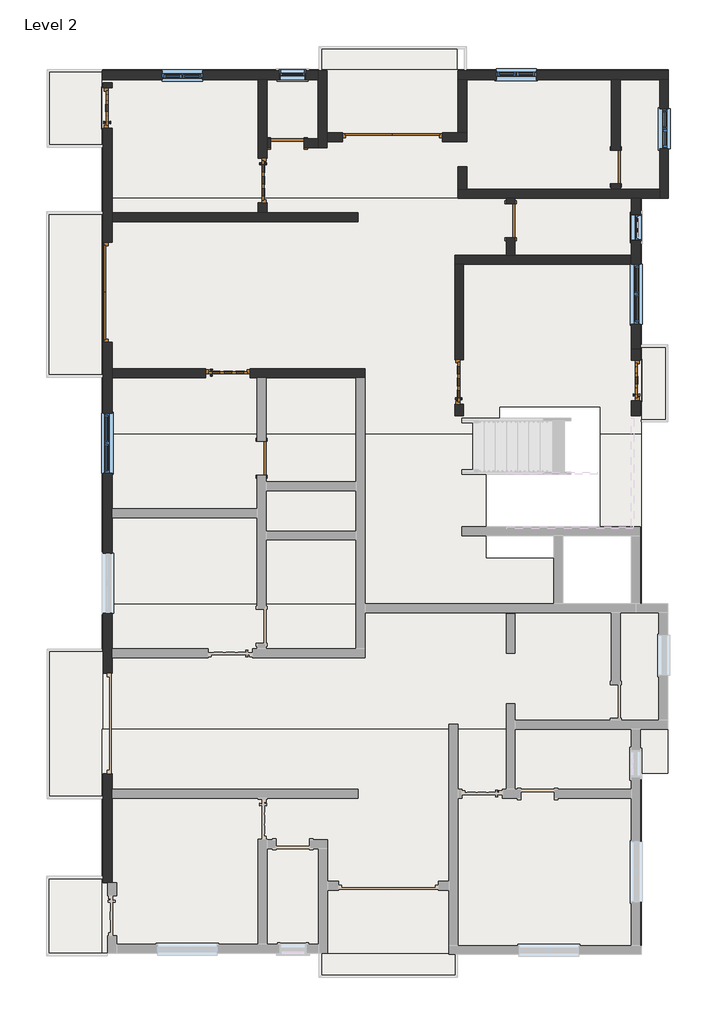
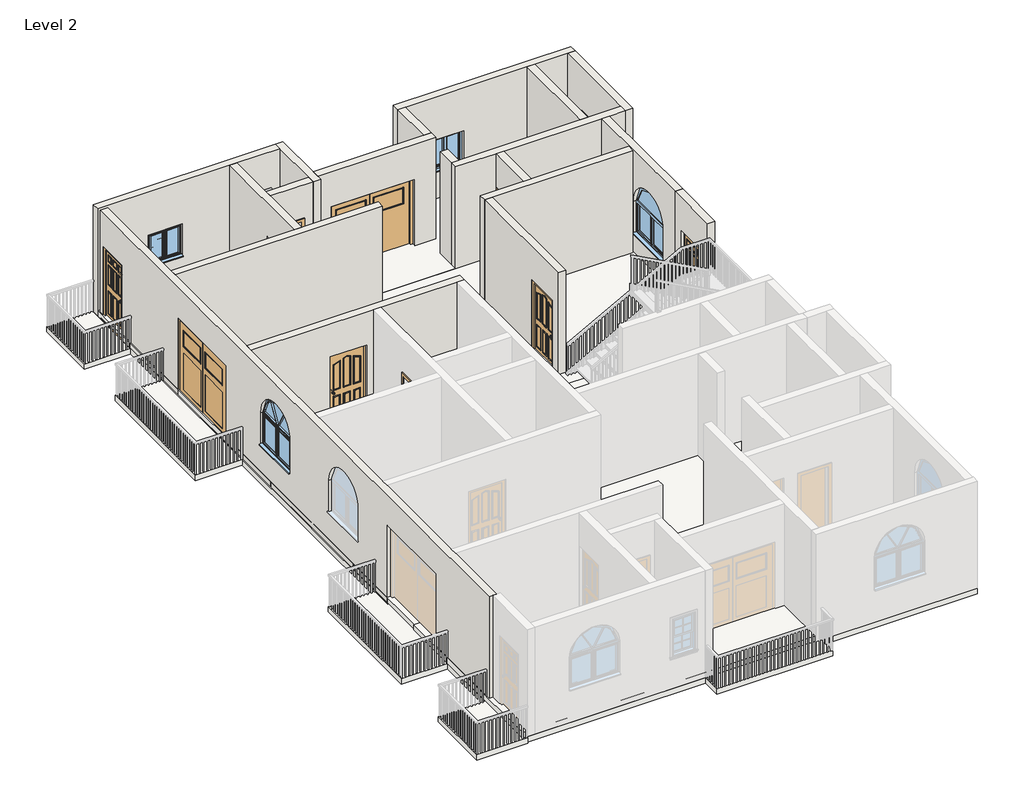
# One storey, part 2 of 7: 19 walls, 11 doors, 10 slabs, 7 windows, 5 roofs.
"""IFC4 building model written with IfcOpenShell, lengths in millimetres."""

from ifc_helpers import new_model, si_unit, point, frame, frame_2d, origin, place, context, project, spatial, polyline, circle_curve, trimmed, segment, composite_curve, outline, extrude, faceted_brep, transform, mapped, element, save
from ifc_brep_helpers import plane_surface, revolved_surface, advanced_brep
from components import doors_extsgl_5_910x2110mm_99758a98, doors_extsgl_5_910x2110mm_d3ca6061, doors_extsgl_6_1010x2110mm_b93c615f, doors_extsgl_6_1010x2110mm_efbaf1af, doors_garage_timber_side_hung_glazing_2270x2050mm_ae99176d, doors_garage_timber_side_hung_glazing_2270x2200mm_badb7014, door_53b1b562, window_679d2811, windows_arched_1360x910mm_c5754810, windows_dbl_w_glazing_bars_910x910mm_41eba874

model = new_model("IFC4")

# Units and contexts
model_context = context("Model", 3, world=origin())
ifc_project = project(units=[si_unit("LENGTHUNIT", "METRE", prefix="MILLI")], contexts=[model_context])

# Site, building, storey
site = spatial("IfcSite", under=ifc_project)
building = spatial("IfcBuilding", under=site)
storey = spatial("IfcBuildingStorey", under=building, Name="Level 2", Elevation=3048.0)

# Doors
placement = place(None, origin())
doors_extsgl_5_910x2110mm_shape = doors_extsgl_5_910x2110mm_99758a98(model_context)
element("IfcDoor", 1, ObjectType="Doors_ExtSgl_5 : 910x2110mm", at=placement, inside=storey, context=model_context, shape_type="MappedRepresentation", body=[
    mapped(doors_extsgl_5_910x2110mm_shape, transform((5761.5890963, 2376.5107951, 3048.0), x_axis=(0.0, 1.0, 0.0), y_axis=(-1.0, 0.0, 0.0), z_axis=(0.0, 0.0, 1.0))),
])
doors_extsgl_5_910x2110mm_2_shape = doors_extsgl_5_910x2110mm_d3ca6061(model_context)
element("IfcDoor", 2, ObjectType="Doors_ExtSgl_5 : 910x2110mm", at=placement, inside=storey, context=model_context, shape_type="MappedRepresentation", body=[
    mapped(doors_extsgl_5_910x2110mm_2_shape, transform((-6229.2013636, 8553.74399, 3048.0), x_axis=(0.0, 1.0, 0.0), y_axis=(-1.0, 0.0, 0.0), z_axis=(0.0, 0.0, 1.0))),
])
doors_extsgl_6_1010x2110mm_shape = doors_extsgl_6_1010x2110mm_b93c615f(model_context)
doors_extsgl_6_1010x2110mm_2_shape = doors_extsgl_6_1010x2110mm_efbaf1af(model_context)
element("IfcDoor", 3, ObjectType="Doors_ExtSgl_6 : 1010x2110mm", at=placement, inside=storey, context=model_context, shape_type="MappedRepresentation", body=[
    mapped(doors_extsgl_6_1010x2110mm_shape, transform((-2709.3109037, 6913.1295584, 3048.0), x_axis=(0.0, -1.0, 0.0), y_axis=(1.0, 0.0, 0.0), z_axis=(0.0, 0.0, 1.0))),
    mapped(doors_extsgl_6_1010x2110mm_2_shape, transform((-2709.3109037, 6913.1295584, 3048.0), x_axis=(0.0, -1.0, 0.0), y_axis=(1.0, 0.0, 0.0), z_axis=(0.0, 0.0, 1.0))),
])
element("IfcDoor", 4, ObjectType="Doors_ExtSgl_6 : 1010x2110mm", at=placement, inside=storey, context=model_context, shape_type="MappedRepresentation", body=[
    mapped(doors_extsgl_6_1010x2110mm_shape, transform((1748.3890963, 2341.0628918, 3048.0), x_axis=(0.0, 1.0, 0.0), y_axis=(-1.0, 0.0, 0.0), z_axis=(0.0, 0.0, 1.0))),
    mapped(doors_extsgl_6_1010x2110mm_2_shape, transform((1748.3890963, 2341.0628918, 3048.0), x_axis=(0.0, 1.0, 0.0), y_axis=(-1.0, 0.0, 0.0), z_axis=(0.0, 0.0, 1.0))),
])
element("IfcDoor", 5, ObjectType="Doors_ExtSgl_6 : 1010x2110mm", at=placement, inside=storey, context=model_context, shape_type="MappedRepresentation", body=[
    mapped(doors_extsgl_6_1010x2110mm_shape, transform((-3496.7442371, 2544.2962251, 3048.0), x_axis=(1.0, 0.0, 0.0), y_axis=(0.0, 1.0, 0.0), z_axis=(0.0, 0.0, 1.0))),
    mapped(doors_extsgl_6_1010x2110mm_2_shape, transform((-3496.7442371, 2544.2962251, 3048.0), x_axis=(1.0, 0.0, 0.0), y_axis=(0.0, 1.0, 0.0), z_axis=(0.0, 0.0, 1.0))),
])
doors_garage_timber_side_hung_glazing_2270x2050mm_shape = doors_garage_timber_side_hung_glazing_2270x2050mm_ae99176d(model_context)
element("IfcDoor", 6, ObjectType="Doors_Garage_Timber_Side_Hung_Glazing : 2270x2050mm", at=placement, inside=storey, context=model_context, shape_type="MappedRepresentation", body=[
    mapped(doors_garage_timber_side_hung_glazing_2270x2050mm_shape, transform((237.0890963, 7890.9962251, 3048.0), x_axis=(1.0, 0.0, 0.0), y_axis=(0.0, 1.0, 0.0), z_axis=(0.0, 0.0, 1.0))),
])
doors_garage_timber_side_hung_glazing_2270x2200mm_shape = doors_garage_timber_side_hung_glazing_2270x2200mm_badb7014(model_context)
element("IfcDoor", 7, ObjectType="Doors_Garage_Timber_Side_Hung_Glazing : 2270x2200mm", at=placement, inside=storey, context=model_context, shape_type="MappedRepresentation", body=[
    mapped(doors_garage_timber_side_hung_glazing_2270x2200mm_shape, transform((-6229.2013636, 4373.0962251, 3048.0), x_axis=(0.0, -1.0, 0.0), y_axis=(1.0, 0.0, 0.0), z_axis=(0.0, 0.0, 1.0))),
])
door_shape = door_53b1b562(model_context)
element("IfcDoor", 8, ObjectType="Single-Flush : 30\" x 80\"", at=placement, inside=storey, context=model_context, shape_type="MappedRepresentation", body=[
    mapped(door_shape, transform((-2150.5109037, 7751.2962251, 3048.0), x_axis=(-1.0, 0.0, 0.0), y_axis=(0.0, -1.0, 0.0), z_axis=(0.0, 0.0, 1.0))),
])
element("IfcDoor", 9, ObjectType="Single-Flush : 30\" x 80\"", at=placement, inside=storey, context=model_context, shape_type="MappedRepresentation", body=[
    mapped(door_shape, transform((2916.7890963, 5998.6962251, 3048.0), x_axis=(0.0, 1.0, 0.0), y_axis=(-1.0, 0.0, 0.0), z_axis=(0.0, 0.0, 1.0))),
])
element("IfcDoor", 10, ObjectType="Single-Flush : 30\" x 80\"", at=placement, inside=storey, context=model_context, shape_type="MappedRepresentation", body=[
    mapped(door_shape, transform((-2734.7109037, 613.8962251, 3048.0), x_axis=(0.0, 1.0, 0.0), y_axis=(-1.0, 0.0, 0.0), z_axis=(0.0, 0.0, 1.0))),
])
element("IfcDoor", 11, ObjectType="Single-Flush : 30\" x 80\"", at=placement, inside=storey, context=model_context, shape_type="MappedRepresentation", body=[
    mapped(door_shape, transform((5304.3890963, 7217.8962251, 3048.0), x_axis=(0.0, 1.0, 0.0), y_axis=(-1.0, 0.0, 0.0), z_axis=(0.0, 0.0, 1.0))),
])

# Roofs
element("IfcRoof", 12, ObjectType="Generic - 12\"", at=placement, inside=storey, context=model_context, shape_type="SweptSolid", body=[
    extrude(outline(polyline([(-6354.2109037, 9427.2527313), (6498.1890963, 9427.2527313), (6498.1890963, 6506.6962251), (-6354.2109037, 6506.6962251), (-6354.2109037, 9427.2527313)])), frame((0.0, 0.0, 3048.0), z_axis=(0.0, 0.0, 1.0), x_axis=(1.0, 0.0, 0.0)), (0.0, 0.0, 1.0), 152.4),
])
element("IfcRoof", 13, ObjectType="Generic - 12\"", at=placement, inside=storey, context=model_context, shape_type="SweptSolid", body=[
    extrude(outline(polyline([(-6330.8013636, -2688.1037749), (6485.4890963, -2688.1037749), (6485.4890963, -6529.1251987), (-6330.8013636, -6529.1251987), (-6330.8013636, -2688.1037749)])), frame((0.0, 0.0, 3048.0), z_axis=(0.0, 0.0, 1.0), x_axis=(1.0, 0.0, 0.0)), (0.0, 0.0, 1.0), 152.4),
])
element("IfcRoof", 14, ObjectType="Generic - 12\"", at=placement, inside=storey, context=model_context, shape_type="SweptSolid", body=[
    extrude(outline(polyline([(-6354.2109037, -5532.9037749), (5863.1890963, -5532.9037749), (5863.1890963, -10612.9037749), (-6354.2109037, -10612.9037749), (-6354.2109037, -5532.9037749)])), frame((0.0, 0.0, 3048.0), z_axis=(0.0, 0.0, 1.0), x_axis=(1.0, 0.0, 0.0)), (0.0, 0.0, 1.0), 152.4),
])
element("IfcRoof", 15, ObjectType="Generic - 12\"", at=placement, inside=storey, context=model_context, shape_type="SweptSolid", body=[
    extrude(outline(polyline([(-6330.8013636, 1160.801054), (-6330.8013636, 6506.6962251), (5875.8890963, 6506.6962251), (5875.8890963, 1160.801054), (4949.8616623, 1160.801054), (4949.8616623, 1784.6684315), (2663.8616623, 1784.6684315), (2663.8616623, 1160.801054), (-6330.8013636, 1160.801054)])), frame((0.0, 0.0, 3048.0), z_axis=(0.0, 0.0, 1.0), x_axis=(1.0, 0.0, 0.0)), (0.0, 0.0, 1.0), 152.4),
])
element("IfcRoof", 16, ObjectType="Generic - 12\"", at=placement, inside=storey, context=model_context, shape_type="SweptSolid", body=[
    extrude(outline(polyline([(-6330.8013636, -2688.1037749), (-6330.8013636, 1160.801054), (2663.8616623, 1160.801054), (2663.8616623, 941.43649), (2352.8853127, 941.43649), (2352.8853127, -1649.36351), (4097.8890963, -1649.36351), (4097.8890963, -2688.1037749), (-6330.8013636, -2688.1037749)])), frame((0.0, 0.0, 3048.0), z_axis=(0.0, 0.0, 1.0), x_axis=(1.0, 0.0, 0.0)), (0.0, 0.0, 1.0), 152.4),
    extrude(outline(polyline([(5875.8890963, 1160.801054), (5875.8890963, -2688.1037749), (5659.9890963, -2688.1037749), (5659.9890963, -1138.7037749), (4791.2853127, -1138.7037749), (4791.2853127, -958.5315685), (4949.8616623, -958.5315685), (4949.8616623, 1160.801054), (5875.8890963, 1160.801054)])), frame((0.0, 0.0, 3048.0), z_axis=(0.0, 0.0, 1.0), x_axis=(1.0, 0.0, 0.0)), (0.0, 0.0, 1.0), 152.4),
])

# Slabs
element("IfcSlab", 17, ObjectType="Generic - 12\"", at=placement, inside=storey, context=model_context, shape_type="SweptSolid", body=[
    extrude(outline(polyline([(1694.4140963, 9948.3962251), (1694.4140963, -11133.6037749), (-1426.6109037, -11133.6037749), (-1426.6109037, 9948.3962251), (1694.4140963, 9948.3962251)])), frame((0.0, 0.0, 2895.6), z_axis=(0.0, 0.0, 1.0), x_axis=(1.0, 0.0, 0.0)), (0.0, 0.0, 1.0), 152.4),
])
element("IfcSlab", 18, ObjectType="Generic - 12\"", at=placement, inside=storey, context=model_context, shape_type="SweptSolid", body=[
    extrude(outline(polyline([(5875.8890963, 9402.2962251), (5875.8890963, -10638.3037749), (1722.9890963, -10638.3037749), (1722.9890963, 9402.2962251), (5875.8890963, 9402.2962251)]), holes=[polyline([(4097.8890963, -2688.1037749), (5659.9890963, -2688.1037749), (5659.9890963, -1138.7037749), (4791.2853127, -1138.7037749), (4791.2853127, -958.5315685), (4949.8616623, -958.5315685), (4949.8616623, 1784.6684315), (2663.8616623, 1784.6684315), (2663.8616623, 941.43649), (2352.8853127, 941.43649), (2352.8853127, -1649.36351), (4097.8890963, -1649.36351), (4097.8890963, -2688.1037749)])]), frame((0.0, 0.0, 2895.6), z_axis=(0.0, 0.0, 1.0), x_axis=(1.0, 0.0, 0.0)), (0.0, 0.0, 1.0), 152.4),
])
element("IfcSlab", 19, ObjectType="Generic - 12\"", at=placement, inside=storey, context=model_context, shape_type="SweptSolid", body=[
    extrude(outline(polyline([(6498.1890963, 9402.2962251), (6498.1890963, 6506.6962251), (5875.8890963, 6506.6962251), (5875.8890963, 9402.2962251), (6498.1890963, 9402.2962251)])), frame((0.0, 0.0, 2895.6), z_axis=(0.0, 0.0, 1.0), x_axis=(1.0, 0.0, 0.0)), (0.0, 0.0, 1.0), 152.4),
])
element("IfcSlab", 20, ObjectType="Generic - 12\"", at=placement, inside=storey, context=model_context, shape_type="SweptSolid", body=[
    extrude(outline(polyline([(6485.4890963, 3183.81308), (6485.4890963, 1439.3962251), (5863.1890963, 1439.3962251), (5863.1890963, 3183.81308), (6485.4890963, 3183.81308)])), frame((0.0, 0.0, 2895.6), z_axis=(0.0, 0.0, 1.0), x_axis=(1.0, 0.0, 0.0)), (0.0, 0.0, 1.0), 152.4),
])
element("IfcSlab", 21, ObjectType="Generic - 12\"", at=placement, inside=storey, context=model_context, shape_type="SweptSolid", body=[
    extrude(outline(polyline([(6485.4890963, -2688.1037749), (6485.4890963, -5532.9037749), (5863.1890963, -5532.9037749), (5863.1890963, -2688.1037749), (6485.4890963, -2688.1037749)])), frame((0.0, 0.0, 2895.6), z_axis=(0.0, 0.0, 1.0), x_axis=(1.0, 0.0, 0.0)), (0.0, 0.0, 1.0), 152.4),
])
element("IfcSlab", 22, ObjectType="Generic - 12\"", at=placement, inside=storey, context=model_context, shape_type="SweptSolid", body=[
    extrude(outline(polyline([(-6330.8013636, 9427.2527313), (-6330.8013636, 7667.1584215), (-7598.8109037, 7667.1584215), (-7598.8109037, 9427.2527313), (-6330.8013636, 9427.2527313)])), frame((0.0, 0.0, 2895.6), z_axis=(0.0, 0.0, 1.0), x_axis=(1.0, 0.0, 0.0)), (0.0, 0.0, 1.0), 152.4),
])
element("IfcSlab", 23, ObjectType="Generic - 12\"", at=placement, inside=storey, context=model_context, shape_type="SweptSolid", body=[
    extrude(outline(polyline([(-6330.8013636, 6201.8962251), (-6330.8013636, 2455.3962251), (-7614.6859037, 2455.3962251), (-7614.6859037, 6201.8962251), (-6330.8013636, 6201.8962251)])), frame((0.0, 0.0, 2895.6), z_axis=(0.0, 0.0, 1.0), x_axis=(1.0, 0.0, 0.0)), (0.0, 0.0, 1.0), 152.4),
])
element("IfcSlab", 24, ObjectType="Generic - 12\"", at=placement, inside=storey, context=model_context, shape_type="SweptSolid", body=[
    extrude(outline(polyline([(-6330.8013636, -3716.8037749), (-6330.8013636, -7105.2894702), (-7598.8109037, -7105.2894702), (-7598.8109037, -3716.8037749), (-6330.8013636, -3716.8037749)])), frame((0.0, 0.0, 2895.6), z_axis=(0.0, 0.0, 1.0), x_axis=(1.0, 0.0, 0.0)), (0.0, 0.0, 1.0), 152.4),
])
element("IfcSlab", 25, ObjectType="Generic - 12\"", at=placement, inside=storey, context=model_context, shape_type="SweptSolid", body=[
    extrude(outline(polyline([(-6243.0859037, -8868.0845215), (-6243.0859037, -10663.7037749), (-7614.6859037, -10663.7037749), (-7614.6859037, -8868.0845215), (-6243.0859037, -8868.0845215)])), frame((0.0, 0.0, 2895.6), z_axis=(0.0, 0.0, 1.0), x_axis=(1.0, 0.0, 0.0)), (0.0, 0.0, 1.0), 152.4),
])
element("IfcSlab", 26, ObjectType="Generic - 12\"", at=placement, inside=storey, context=model_context, shape_type="SweptSolid", body=[
    extrude(outline(polyline([(-1236.1109037, 9427.2527313), (-1236.1109037, -10612.9037749), (-6354.2109037, -10612.9037749), (-6354.2109037, 9427.2527313), (-1236.1109037, 9427.2527313)])), frame((0.0, 0.0, 2895.6), z_axis=(0.0, 0.0, 1.0), x_axis=(1.0, 0.0, 0.0)), (0.0, 0.0, 1.0), 152.4),
])

# Walls
element("IfcWall", 27, ObjectType="Generic - 9\" w", at=placement, inside=storey, context=model_context, shape_type="Brep", body=[
    faceted_brep([(1722.9890963, 9199.0962251, 3048.0), (1926.1890963, 9199.0962251, 3048.0), (5202.7890963, 9199.0962251, 3048.0), (5405.9890963, 9199.0962251, 3048.0), (6294.9890963, 9199.0962251, 3048.0), (6498.1890963, 9199.0962251, 3048.0), (6498.1890963, 9199.0962251, 6096.0), (6294.9890963, 9199.0962251, 6096.0), (5405.9890963, 9199.0962251, 6096.0), (5202.7890963, 9199.0962251, 6096.0), (1926.1890963, 9199.0962251, 6096.0), (1722.9890963, 9199.0962251, 6096.0), (2588.7890963, 9199.0962251, 4872.4), (3498.7890963, 9199.0962251, 4872.4), (3498.7890963, 9199.0962251, 3962.4), (2588.7890963, 9199.0962251, 3962.4), (1722.9890963, 9402.2962251, 3048.0), (1722.9890963, 9402.2962251, 6096.0), (6498.1890963, 9402.2962251, 6096.0), (6498.1890963, 9402.2962251, 3048.0), (2588.7890963, 9402.2962251, 4872.4), (2588.7890963, 9402.2962251, 3962.4), (3498.7890963, 9402.2962251, 3962.4), (3498.7890963, 9402.2962251, 4872.4)], [[[0, 1, 2, 3, 4, 5, 6, 7, 8, 9, 10, 11], [12, 13, 14, 15]], [[16, 17, 18, 19], [20, 21, 22, 23]], [[5, 4, 3, 2, 1, 0, 16, 19]], [[11, 10, 9, 8, 7, 6, 18, 17]], [[0, 11, 17, 16]], [[6, 5, 19, 18]], [[21, 20, 12, 15]], [[22, 21, 15, 14]], [[23, 22, 14, 13]], [[20, 23, 13, 12]]]),
])
element("IfcWall", 28, ObjectType="Generic - 9\" w", at=placement, inside=storey, context=model_context, shape_type="SweptSolid", body=[
    extrude(outline(polyline([(6506.6962251, 3048.0), (3087.7441284, 3048.0), (3087.7441284, 6096.0), (6506.6962251, 6096.0), (6506.6962251, 3048.0)]), holes=[polyline([(6151.0962251, 5029.2), (5541.4962251, 5029.2), (5541.4962251, 3962.4), (6151.0962251, 3962.4), (6151.0962251, 5029.2)]), composite_curve([segment(polyline([(5016.7786331, 3733.6617803), (5016.7786331, 4643.6617803)]), True, "CONTINUOUS"), segment(trimmed(circle_curve(frame_2d((4336.7786331, 4643.6617803)), 680.0), [point((5016.7786331, 4643.6617803))], [point((3656.7786331, 4643.6617803))], True, "CARTESIAN"), True, "CONTINUOUS"), segment(polyline([(3656.7786331, 4643.6617803), (3656.7786331, 3733.6617803), (5016.7786331, 3733.6617803)]), True, "CONTINUOUS")], self_intersect=False)]), frame((5659.9890963, 0.0, 0.0), z_axis=(1.0, 0.0, 0.0), x_axis=(0.0, 1.0, 0.0)), (0.0, 0.0, 1.0), 203.2),
])
element("IfcWall", 29, ObjectType="Generic - 9\" w", at=placement, inside=storey, context=model_context, shape_type="AdvancedBrep", body=[
    advanced_brep(
    [(-6330.8013636, 3238.0962251, 3048.0), (-6330.8013636, -4267.1251987, 3048.0), (-6330.8013636, -4267.1251987, 5248.0), (-6330.8013636, -6537.1251987, 5248.0), (-6330.8013636, -6537.1251987, 3048.0), (-6330.8013636, -9007.7845215, 3048.0), (-6330.8013636, -9007.7845215, 6096.0), (-6330.8013636, 9129.8816143, 6096.0), (-6330.8013636, 9129.8816143, 3048.0), (-6330.8013636, 9008.7773233, 3048.0), (-6330.8013636, 9008.7773233, 5158.0), (-6330.8013636, 8098.7773233, 5158.0), (-6330.8013636, 8098.7773233, 3048.0), (-6330.8013636, 5508.0962251, 3048.0), (-6330.8013636, 5508.0962251, 5248.0), (-6330.8013636, 3238.0962251, 5248.0), (-6330.8013636, 276.7962251, 3962.4), (-6330.8013636, 1636.7962251, 3962.4), (-6330.8013636, 1636.7962251, 4872.4), (-6330.8013636, 276.7962251, 4872.4), (-6330.8013636, -1538.2037749, 3962.4), (-6330.8013636, -1538.2037749, 4872.4), (-6330.8013636, -2898.2037749, 4872.4), (-6330.8013636, -2898.2037749, 3962.4), (-6127.6013636, -4267.1251987, 5248.0), (-6127.6013636, -4267.1251987, 3048.0), (-6127.6013636, -3907.3037749, 3048.0), (-6127.6013636, -3704.1037749, 3048.0), (-6127.6013636, -732.3037749, 3048.0), (-6127.6013636, -529.1037749, 3048.0), (-6127.6013636, 2442.6962251, 3048.0), (-6127.6013636, 2645.8962251, 3048.0), (-6127.6013636, 3238.0962251, 3048.0), (-6127.6013636, 3238.0962251, 5248.0), (-6127.6013636, 5508.0962251, 5248.0), (-6127.6013636, 5508.0962251, 3048.0), (-6127.6013636, 5973.2962251, 3048.0), (-6127.6013636, 6176.4962251, 3048.0), (-6127.6013636, 8098.7773233, 3048.0), (-6127.6013636, 8098.7773233, 5158.0), (-6127.6013636, 9008.7773233, 5158.0), (-6127.6013636, 9008.7773233, 3048.0), (-6127.6013636, 9129.8816143, 3048.0), (-6127.6013636, 9129.8816143, 6096.0), (-6127.6013636, 6176.4962251, 6096.0), (-6127.6013636, 5973.2962251, 6096.0), (-6127.6013636, 2645.8962251, 6096.0), (-6127.6013636, 2442.6962251, 6096.0), (-6127.6013636, -529.1037749, 6096.0), (-6127.6013636, -732.3037749, 6096.0), (-6127.6013636, -3704.1037749, 6096.0), (-6127.6013636, -3907.3037749, 6096.0), (-6127.6013636, -6896.9466225, 6096.0), (-6127.6013636, -7100.1466225, 6096.0), (-6127.6013636, -9007.7845215, 6096.0), (-6127.6013636, -9007.7845215, 3048.0), (-6127.6013636, -7100.1466225, 3048.0), (-6127.6013636, -6896.9466225, 3048.0), (-6127.6013636, -6537.1251987, 3048.0), (-6127.6013636, -6537.1251987, 5248.0), (-6127.6013636, 276.7962251, 3962.4), (-6127.6013636, 276.7962251, 4872.4), (-6127.6013636, 1636.7962251, 4872.4), (-6127.6013636, 1636.7962251, 3962.4), (-6127.6013636, -1538.2037749, 3962.4), (-6127.6013636, -2898.2037749, 3962.4), (-6127.6013636, -2898.2037749, 4872.4), (-6127.6013636, -1538.2037749, 4872.4), (-6229.2013636, -9007.7845215, 3048.0), (-6229.2013636, -9007.7845215, 6096.0)],
    [
        (0, 1),
        (1, 2),
        (2, 3),
        (3, 4),
        (4, 5),
        (5, 6),
        (6, 7),
        (7, 8),
        (8, 9),
        (9, 10),
        (10, 11),
        (11, 12),
        (12, 13),
        (13, 14),
        (14, 15),
        (15, 0),
        (16, 17),
        (17, 18),
        (18, 19, circle_curve(frame((-6330.8013636, 956.7962251, 4872.4), z_axis=(1.0, 0.0, 0.0), x_axis=(0.0, 1.0, 0.0)), 680.0)),
        (19, 16),
        (20, 21),
        (21, 22, circle_curve(frame((-6330.8013636, -2218.2037749, 4872.4), z_axis=(1.0, 0.0, 0.0), x_axis=(0.0, -1.0, 0.0)), 680.0)),
        (22, 23),
        (23, 20),
        (24, 25),
        (25, 26),
        (26, 27),
        (27, 28),
        (28, 29),
        (29, 30),
        (30, 31),
        (31, 32),
        (32, 33),
        (33, 34),
        (34, 35),
        (35, 36),
        (36, 37),
        (37, 38),
        (38, 39),
        (39, 40),
        (40, 41),
        (41, 42),
        (42, 43),
        (43, 44),
        (44, 45),
        (45, 46),
        (46, 47),
        (47, 48),
        (48, 49),
        (49, 50),
        (50, 51),
        (51, 52),
        (52, 53),
        (53, 54),
        (54, 55),
        (55, 56),
        (56, 57),
        (57, 58),
        (58, 59),
        (59, 24),
        (60, 61),
        (61, 62, circle_curve(frame((-6127.6013636, 956.7962251, 4872.4), z_axis=(-1.0, 0.0, 0.0), x_axis=(0.0, 1.0, 0.0)), 680.0)),
        (62, 63),
        (63, 60),
        (64, 65),
        (65, 66),
        (66, 67, circle_curve(frame((-6127.6013636, -2218.2037749, 4872.4), z_axis=(-1.0, 0.0, 0.0), x_axis=(0.0, -1.0, 0.0)), 680.0)),
        (67, 64),
        (41, 9),
        (8, 42),
        (12, 38),
        (35, 13),
        (55, 68),
        (68, 5),
        (4, 58),
        (25, 1),
        (0, 32),
        (54, 69),
        (69, 6),
        (43, 7),
        (11, 39),
        (40, 10),
        (34, 14),
        (15, 33),
        (3, 59),
        (24, 2),
        (60, 16),
        (19, 61),
        (18, 62),
        (17, 63),
        (20, 64),
        (67, 21),
        (66, 22),
        (65, 23),
    ],
    [
        plane_surface(frame((-6330.8013636, 2442.6962251, 3048.0), z_axis=(-1.0, 0.0, 0.0), x_axis=(0.0, -1.0, 0.0))),
        plane_surface(frame((-6127.6013636, 2442.6962251, 3048.0), z_axis=(1.0, 0.0, 0.0), x_axis=(0.0, 1.0, 0.0))),
        plane_surface(frame((-6330.8013636, 9129.8816143, 3048.0), z_axis=(0.0, 0.0, -1.0), x_axis=(1.0, 0.0, 0.0))),
        plane_surface(frame((-6330.8013636, -9007.7845215, 3048.0), z_axis=(0.0, -1.0, 0.0), x_axis=(1.0, 0.0, 0.0))),
        plane_surface(frame((-6330.8013636, -9007.7845215, 6096.0), z_axis=(0.0, 0.0, 1.0), x_axis=(1.0, 0.0, 0.0))),
        plane_surface(frame((-6330.8013636, 9129.8816143, 6096.0), z_axis=(0.0, 1.0, 0.0), x_axis=(1.0, 0.0, 0.0))),
        plane_surface(frame((-6330.8013636, 8098.7773233, 5158.0), z_axis=(0.0, 1.0, 0.0), x_axis=(1.0, 0.0, 0.0))),
        plane_surface(frame((-6330.8013636, 9008.7773233, 3048.0), z_axis=(0.0, -1.0, 0.0), x_axis=(1.0, 0.0, 0.0))),
        plane_surface(frame((-6330.8013636, 9008.7773233, 5158.0), z_axis=(0.0, 0.0, -1.0), x_axis=(1.0, 0.0, 0.0))),
        plane_surface(frame((-6127.6013636, 5508.0962251, 5248.0), z_axis=(0.0, -1.0, 0.0), x_axis=(-1.0, 0.0, 0.0))),
        plane_surface(frame((-6127.6013636, 3238.0962251, 3048.0), z_axis=(0.0, 1.0, 0.0), x_axis=(-1.0, 0.0, 0.0))),
        plane_surface(frame((-6127.6013636, 3238.0962251, 5248.0), z_axis=(0.0, 0.0, -1.0), x_axis=(-1.0, 0.0, 0.0))),
        plane_surface(frame((-6330.8013636, -6537.1251987, 5248.0), z_axis=(0.0, 1.0, 0.0), x_axis=(1.0, 0.0, 0.0))),
        plane_surface(frame((-6330.8013636, -4267.1251987, 3048.0), z_axis=(0.0, -1.0, 0.0), x_axis=(1.0, 0.0, 0.0))),
        plane_surface(frame((-6330.8013636, -4267.1251987, 5248.0), z_axis=(0.0, 0.0, -1.0), x_axis=(1.0, 0.0, 0.0))),
        plane_surface(frame((-6127.6013636, 276.7962251, 3962.4), z_axis=(0.0, 1.0, 0.0), x_axis=(-1.0, 0.0, 0.0))),
        revolved_surface(polyline([(-6330.8013636, 1636.7962251, 4872.4), (-6127.6013636, 1636.7962251, 4872.4)]), (-6127.6013636, 956.7962251, 4872.4), (-1.0, 0.0, 0.0)),
        plane_surface(frame((-6127.6013636, 1636.7962251, 4872.4), z_axis=(0.0, -1.0, 0.0), x_axis=(-1.0, 0.0, 0.0))),
        plane_surface(frame((-6127.6013636, 1636.7962251, 3962.4), z_axis=(0.0, 0.0, 1.0), x_axis=(-1.0, 0.0, 0.0))),
        plane_surface(frame((-6330.8013636, -1538.2037749, 3962.4), z_axis=(0.0, -1.0, 0.0), x_axis=(1.0, 0.0, 0.0))),
        revolved_surface(polyline([(-6127.6013636, -2898.2037749, 4872.4), (-6330.8013636, -2898.2037749, 4872.4)]), (-6330.8013636, -2218.2037749, 4872.4), (1.0, 0.0, 0.0)),
        plane_surface(frame((-6330.8013636, -2898.2037749, 4872.4), z_axis=(0.0, 1.0, 0.0), x_axis=(1.0, 0.0, 0.0))),
        plane_surface(frame((-6330.8013636, -2898.2037749, 3962.4), z_axis=(0.0, 0.0, 1.0), x_axis=(1.0, 0.0, 0.0))),
    ],
    [
        (0, [[1, 2, 3, 4, 5, 6, 7, 8, 9, 10, 11, 12, 13, 14, 15, 16], [17, 18, 19, 20], [21, 22, 23, 24]]),
        (1, [[25, 26, 27, 28, 29, 30, 31, 32, 33, 34, 35, 36, 37, 38, 39, 40, 41, 42, 43, 44, 45, 46, 47, 48, 49, 50, 51, 52, 53, 54, 55, 56, 57, 58, 59, 60], [61, 62, 63, 64], [65, 66, 67, 68]]),
        (2, [[-42, 69, -9, 70]]),
        (2, [[-13, 71, -38, -37, -36, 72]]),
        (2, [[-58, -57, -56, 73, 74, -5, 75]]),
        (2, [[-32, -31, -30, -29, -28, -27, -26, 76, -1, 77]]),
        (3, [[-6, -74, -73, -55, 78, 79]]),
        (4, [[-7, -79, -78, -54, -53, -52, -51, -50, -49, -48, -47, -46, -45, -44, 80]]),
        (5, [[-8, -80, -43, -70]]),
        (6, [[-12, 81, -39, -71]]),
        (7, [[-10, -69, -41, 82]]),
        (8, [[-11, -82, -40, -81]]),
        (9, [[-35, 83, -14, -72]]),
        (10, [[-33, -77, -16, 84]]),
        (11, [[-34, -84, -15, -83]]),
        (12, [[-4, 85, -59, -75]]),
        (13, [[-2, -76, -25, 86]]),
        (14, [[-3, -86, -60, -85]]),
        (15, [[-61, 87, -20, 88]]),
        (16, [[-62, -88, -19, 89]]),
        (17, [[-63, -89, -18, 90]]),
        (18, [[-64, -90, -17, -87]]),
        (19, [[-21, 91, -68, 92]]),
        (20, [[-22, -92, -67, 93]]),
        (21, [[-23, -93, -66, 94]]),
        (22, [[-24, -94, -65, -91]]),
    ],
),
])
element("IfcWall", 30, ObjectType="Generic - 9\" w", at=placement, inside=storey, context=model_context, shape_type="SweptSolid", body=[
    extrude(outline(polyline([(3087.7441284, 3048.0), (2831.5441284, 3048.0), (2831.5441284, 5158.0), (1921.5441284, 5158.0), (1921.5441284, 3048.0), (1579.0962251, 3048.0), (1579.0962251, 6096.0), (3087.7441284, 6096.0), (3087.7441284, 3048.0)])), frame((5659.9890963, 0.0, 0.0), z_axis=(1.0, 0.0, 0.0), x_axis=(0.0, 1.0, 0.0)), (0.0, 0.0, 1.0), 203.2),
])
element("IfcWall", 31, ObjectType="Generic - 9\" w", at=placement, inside=storey, context=model_context, shape_type="Brep", body=[
    faceted_brep([(-1452.0109037, 9401.8527313, 3048.0), (-6354.2109037, 9401.8527313, 3048.0), (-6354.2109037, 9401.8527313, 6096.0), (-1452.0109037, 9401.8527313, 6096.0), (-4076.7609037, 9401.8527313, 4872.4), (-4986.7609037, 9401.8527313, 4872.4), (-4986.7609037, 9401.8527313, 3962.4), (-4076.7609037, 9401.8527313, 3962.4), (-2334.6609037, 9401.8527313, 5029.2), (-2334.6609037, 9401.8527313, 3962.4), (-1725.0609037, 9401.8527313, 3962.4), (-1725.0609037, 9401.8527313, 5029.2), (-1452.0109037, 9198.6527313, 3048.0), (-1452.0109037, 9198.6527313, 6096.0), (-2607.7109037, 9198.6527313, 6096.0), (-2810.9109037, 9198.6527313, 6096.0), (-6354.2109037, 9198.6527313, 6096.0), (-6354.2109037, 9198.6527313, 3048.0), (-2810.9109037, 9198.6527313, 3048.0), (-2607.7109037, 9198.6527313, 3048.0), (-4076.7609037, 9198.6527313, 4872.4), (-4076.7609037, 9198.6527313, 3962.4), (-4986.7609037, 9198.6527313, 3962.4), (-4986.7609037, 9198.6527313, 4872.4), (-2334.6609037, 9198.6527313, 5029.2), (-1725.0609037, 9198.6527313, 5029.2), (-1725.0609037, 9198.6527313, 3962.4), (-2334.6609037, 9198.6527313, 3962.4)], [[[0, 1, 2, 3], [4, 5, 6, 7], [8, 9, 10, 11]], [[12, 13, 14, 15, 16, 17, 18, 19], [20, 21, 22, 23], [24, 25, 26, 27]], [[1, 0, 12, 19, 18, 17]], [[2, 1, 17, 16]], [[3, 2, 16, 15, 14, 13]], [[0, 3, 13, 12]], [[21, 20, 4, 7]], [[22, 21, 7, 6]], [[23, 22, 6, 5]], [[20, 23, 5, 4]], [[9, 8, 24, 27]], [[10, 9, 27, 26]], [[11, 10, 26, 25]], [[8, 11, 25, 24]]]),
])
element("IfcWall", 32, ObjectType="Generic -4.5\" p", at=placement, inside=storey, context=model_context, shape_type="Brep", body=[
    faceted_brep([(-2810.9109037, 6408.0962251, 5158.0), (-2810.9109037, 6408.0962251, 3048.0), (-2810.9109037, 6176.4962251, 3048.0), (-2810.9109037, 6176.4962251, 6096.0), (-2810.9109037, 9198.6527313, 6096.0), (-2810.9109037, 9198.6527313, 3048.0), (-2810.9109037, 7418.0962251, 3048.0), (-2810.9109037, 7418.0962251, 5158.0), (-2607.7109037, 6176.4962251, 3048.0), (-2607.7109037, 6408.0962251, 3048.0), (-2607.7109037, 6408.0962251, 5158.0), (-2607.7109037, 7418.0962251, 5158.0), (-2607.7109037, 7418.0962251, 3048.0), (-2607.7109037, 7649.6962251, 3048.0), (-2607.7109037, 7852.8962251, 3048.0), (-2607.7109037, 9198.6527313, 3048.0), (-2607.7109037, 9198.6527313, 6096.0), (-2607.7109037, 7852.8962251, 6096.0), (-2607.7109037, 7649.6962251, 6096.0), (-2607.7109037, 6176.4962251, 6096.0)], [[[0, 1, 2, 3, 4, 5, 6, 7]], [[8, 9, 10, 11, 12, 13, 14, 15, 16, 17, 18, 19]], [[6, 5, 15, 14, 13, 12]], [[2, 1, 9, 8]], [[4, 3, 19, 18, 17, 16]], [[3, 2, 8, 19]], [[12, 11, 7, 6]], [[10, 9, 1, 0]], [[11, 10, 0, 7]], [[5, 4, 16, 15]]]),
])
element("IfcWall", 33, ObjectType="Generic -4.5\" p", at=placement, inside=storey, context=model_context, shape_type="Brep", body=[
    faceted_brep([(-6127.6013636, 5973.2962251, 3048.0), (-550.3109037, 5973.2962251, 3048.0), (-550.3109037, 5973.2962251, 6096.0), (-6127.6013636, 5973.2962251, 6096.0), (-6127.6013636, 6176.4962251, 3048.0), (-6127.6013636, 6176.4962251, 6096.0), (-2810.9109037, 6176.4962251, 6096.0), (-2607.7109037, 6176.4962251, 6096.0), (-550.3109037, 6176.4962251, 6096.0), (-550.3109037, 6176.4962251, 3048.0), (-2607.7109037, 6176.4962251, 3048.0), (-2810.9109037, 6176.4962251, 3048.0)], [[[0, 1, 2, 3]], [[4, 5, 6, 7, 8, 9, 10, 11]], [[1, 0, 4, 11, 10, 9]], [[2, 1, 9, 8]], [[3, 2, 8, 7, 6, 5]], [[0, 3, 5, 4]]]),
])
element("IfcWall", 34, ObjectType="Generic -4.5\" p", at=placement, inside=storey, context=model_context, shape_type="Brep", body=[
    faceted_brep([(-1452.0109037, 9401.8527313, 3048.0), (-1452.0109037, 9198.6527313, 3048.0), (-1452.0109037, 7852.8962251, 3048.0), (-1452.0109037, 7649.6962251, 3048.0), (-1452.0109037, 7649.6962251, 6096.0), (-1452.0109037, 7852.8962251, 6096.0), (-1452.0109037, 9198.6527313, 6096.0), (-1452.0109037, 9401.8527313, 6096.0), (-1248.8109037, 9401.8527313, 3048.0), (-1248.8109037, 9401.8527313, 6096.0), (-1248.8109037, 7992.5962251, 6096.0), (-1248.8109037, 7789.3962251, 6096.0), (-1248.8109037, 7649.6962251, 6096.0), (-1248.8109037, 7649.6962251, 3048.0), (-1248.8109037, 7789.3962251, 3048.0), (-1248.8109037, 7992.5962251, 3048.0)], [[[0, 1, 2, 3, 4, 5, 6, 7]], [[8, 9, 10, 11, 12, 13, 14, 15]], [[3, 2, 1, 0, 8, 15, 14, 13]], [[7, 6, 5, 4, 12, 11, 10, 9]], [[4, 3, 13, 12]], [[0, 7, 9, 8]]]),
])
element("IfcWall", 35, ObjectType="Generic -4.5\" p", at=placement, inside=storey, context=model_context, shape_type="SweptSolid", body=[
    extrude(outline(polyline([(3048.0, -2607.7109037), (3048.0, -2531.5109037), (5080.0, -2531.5109037), (5080.0, -1769.5109037), (3048.0, -1769.5109037), (3048.0, -1452.0109037), (6096.0, -1452.0109037), (6096.0, -2607.7109037), (3048.0, -2607.7109037)])), frame((0.0, 7649.6962251, 0.0), z_axis=(0.0, 1.0, 0.0), x_axis=(0.0, 0.0, 1.0)), (0.0, 0.0, 1.0), 203.2),
])
element("IfcWall", 36, ObjectType="Generic -4.5\" p", at=placement, inside=storey, context=model_context, shape_type="Brep", body=[
    faceted_brep([(1372.0890963, 7789.3962251, 5098.0), (1372.0890963, 7789.3962251, 3048.0), (1926.1890963, 7789.3962251, 3048.0), (1926.1890963, 7789.3962251, 6096.0), (-1248.8109037, 7789.3962251, 6096.0), (-1248.8109037, 7789.3962251, 3048.0), (-897.9109037, 7789.3962251, 3048.0), (-897.9109037, 7789.3962251, 5098.0), (1926.1890963, 7992.5962251, 3048.0), (1722.9890963, 7992.5962251, 3048.0), (1372.0890963, 7992.5962251, 3048.0), (1372.0890963, 7992.5962251, 5098.0), (-897.9109037, 7992.5962251, 5098.0), (-897.9109037, 7992.5962251, 3048.0), (-1248.8109037, 7992.5962251, 3048.0), (-1248.8109037, 7992.5962251, 6096.0), (1722.9890963, 7992.5962251, 6096.0), (1926.1890963, 7992.5962251, 6096.0)], [[[0, 1, 2, 3, 4, 5, 6, 7]], [[8, 9, 10, 11, 12, 13, 14, 15, 16, 17]], [[6, 5, 14, 13]], [[2, 1, 10, 9, 8]], [[4, 3, 17, 16, 15]], [[5, 4, 15, 14]], [[3, 2, 8, 17]], [[13, 12, 7, 6]], [[11, 10, 1, 0]], [[12, 11, 0, 7]]]),
])
element("IfcWall", 37, ObjectType="Generic -4.5\" p", at=placement, inside=storey, context=model_context, shape_type="SweptSolid", body=[
    extrude(outline(polyline([(1722.9890963, 7992.5962251), (1722.9890963, 9199.0962251), (1926.1890963, 9199.0962251), (1926.1890963, 7992.5962251), (1722.9890963, 7992.5962251)])), frame((0.0, 0.0, 3048.0), z_axis=(0.0, 0.0, 1.0), x_axis=(1.0, 0.0, 0.0)), (0.0, 0.0, 1.0), 3048.0),
])
element("IfcWall", 38, ObjectType="Generic -4.5\" p", at=placement, inside=storey, context=model_context, shape_type="SweptSolid", body=[
    extrude(outline(polyline([(9199.0962251, 3048.0), (7598.8962251, 3048.0), (7598.8962251, 5080.0), (6836.8962251, 5080.0), (6836.8962251, 3048.0), (6709.8962251, 3048.0), (6709.8962251, 6096.0), (9199.0962251, 6096.0), (9199.0962251, 3048.0)])), frame((5202.7890963, 0.0, 0.0), z_axis=(1.0, 0.0, 0.0), x_axis=(0.0, 1.0, 0.0)), (0.0, 0.0, 1.0), 203.2),
])
element("IfcWall", 39, ObjectType="Generic -4.5\" p", at=placement, inside=storey, context=model_context, shape_type="Brep", body=[
    faceted_brep([(6294.9890963, 9199.0962251, 3048.0), (6294.9890963, 6709.8962251, 3048.0), (6294.9890963, 6506.6962251, 3048.0), (6294.9890963, 6506.6962251, 6096.0), (6294.9890963, 6709.8962251, 6096.0), (6294.9890963, 9199.0962251, 6096.0), (6294.9890963, 8536.4962251, 4872.4), (6294.9890963, 7626.4962251, 4872.4), (6294.9890963, 7626.4962251, 3962.4), (6294.9890963, 8536.4962251, 3962.4), (6498.1890963, 9199.0962251, 3048.0), (6498.1890963, 9199.0962251, 6096.0), (6498.1890963, 6506.6962251, 6096.0), (6498.1890963, 6506.6962251, 3048.0), (6498.1890963, 8536.4962251, 4872.4), (6498.1890963, 8536.4962251, 3962.4), (6498.1890963, 7626.4962251, 3962.4), (6498.1890963, 7626.4962251, 4872.4)], [[[0, 1, 2, 3, 4, 5], [6, 7, 8, 9]], [[10, 11, 12, 13], [14, 15, 16, 17]], [[2, 1, 0, 10, 13]], [[5, 4, 3, 12, 11]], [[3, 2, 13, 12]], [[0, 5, 11, 10]], [[15, 14, 6, 9]], [[16, 15, 9, 8]], [[17, 16, 8, 7]], [[14, 17, 7, 6]]]),
])
element("IfcWall", 40, ObjectType="Generic -4.5\" p", at=placement, inside=storey, context=model_context, shape_type="Brep", body=[
    faceted_brep([(6294.9890963, 6709.8962251, 3048.0), (5405.9890963, 6709.8962251, 3048.0), (5202.7890963, 6709.8962251, 3048.0), (1926.1890963, 6709.8962251, 3048.0), (1722.9890963, 6709.8962251, 3048.0), (1722.9890963, 6709.8962251, 6096.0), (1926.1890963, 6709.8962251, 6096.0), (5202.7890963, 6709.8962251, 6096.0), (5405.9890963, 6709.8962251, 6096.0), (6294.9890963, 6709.8962251, 6096.0), (6294.9890963, 6506.6962251, 3048.0), (6294.9890963, 6506.6962251, 6096.0), (5863.1890963, 6506.6962251, 6096.0), (5659.9890963, 6506.6962251, 6096.0), (3018.3890963, 6506.6962251, 6096.0), (2815.1890963, 6506.6962251, 6096.0), (1722.9890963, 6506.6962251, 6096.0), (1722.9890963, 6506.6962251, 3048.0), (2815.1890963, 6506.6962251, 3048.0), (3018.3890963, 6506.6962251, 3048.0), (5659.9890963, 6506.6962251, 3048.0), (5863.1890963, 6506.6962251, 3048.0)], [[[0, 1, 2, 3, 4, 5, 6, 7, 8, 9]], [[10, 11, 12, 13, 14, 15, 16, 17, 18, 19, 20, 21]], [[4, 3, 2, 1, 0, 10, 21, 20, 19, 18, 17]], [[9, 8, 7, 6, 5, 16, 15, 14, 13, 12, 11]], [[0, 9, 11, 10]], [[5, 4, 17, 16]]]),
])
element("IfcWall", 41, ObjectType="Generic -4.5\" p", at=placement, inside=storey, context=model_context, shape_type="SweptSolid", body=[
    extrude(outline(polyline([(1926.1890963, 7221.6524875), (1926.1890963, 6709.8962251), (1722.9890963, 6709.8962251), (1722.9890963, 7221.6524875), (1926.1890963, 7221.6524875)])), frame((0.0, 0.0, 3048.0), z_axis=(0.0, 0.0, 1.0), x_axis=(1.0, 0.0, 0.0)), (0.0, 0.0, 1.0), 3048.0),
])
element("IfcWall", 42, ObjectType="Generic -4.5\" p", at=placement, inside=storey, context=model_context, shape_type="SweptSolid", body=[
    extrude(outline(polyline([(6506.6962251, 3048.0), (6379.6962251, 3048.0), (6379.6962251, 5080.0), (5617.6962251, 5080.0), (5617.6962251, 3048.0), (5211.2962251, 3048.0), (5211.2962251, 6096.0), (6506.6962251, 6096.0), (6506.6962251, 3048.0)])), frame((2815.1890963, 0.0, 0.0), z_axis=(1.0, 0.0, 0.0), x_axis=(0.0, 1.0, 0.0)), (0.0, 0.0, 1.0), 203.2),
])
element("IfcWall", 43, ObjectType="Generic -4.5\" p", at=placement, inside=storey, context=model_context, shape_type="Brep", body=[
    faceted_brep([(5634.5890963, 5211.2962251, 3048.0), (3018.3890963, 5211.2962251, 3048.0), (2815.1890963, 5211.2962251, 3048.0), (1646.7890963, 5211.2962251, 3048.0), (1646.7890963, 5211.2962251, 6096.0), (2815.1890963, 5211.2962251, 6096.0), (3018.3890963, 5211.2962251, 6096.0), (5634.5890963, 5211.2962251, 6096.0), (5634.5890963, 5008.0962251, 3048.0), (5634.5890963, 5008.0962251, 6096.0), (1849.9890963, 5008.0962251, 6096.0), (1646.7890963, 5008.0962251, 6096.0), (1646.7890963, 5008.0962251, 3048.0), (1849.9890963, 5008.0962251, 3048.0)], [[[0, 1, 2, 3, 4, 5, 6, 7]], [[8, 9, 10, 11, 12, 13]], [[3, 2, 1, 0, 8, 13, 12]], [[7, 6, 5, 4, 11, 10, 9]], [[0, 7, 9, 8]], [[4, 3, 12, 11]]]),
])
element("IfcWall", 44, ObjectType="Generic -4.5\" p", at=placement, inside=storey, context=model_context, shape_type="SweptSolid", body=[
    extrude(outline(polyline([(5008.0962251, 3048.0), (2846.0962251, 3048.0), (2846.0962251, 5158.0), (1836.0962251, 5158.0), (1836.0962251, 3048.0), (1579.0962251, 3048.0), (1579.0962251, 6096.0), (5008.0962251, 6096.0), (5008.0962251, 3048.0)])), frame((1646.7890963, 0.0, 0.0), z_axis=(1.0, 0.0, 0.0), x_axis=(0.0, 1.0, 0.0)), (0.0, 0.0, 1.0), 203.2),
])
element("IfcWall", 45, ObjectType="Generic -4.5\" p", at=placement, inside=storey, context=model_context, shape_type="Brep", body=[
    faceted_brep([(-2991.7109037, 2442.6962251, 5158.0), (-2991.7109037, 2442.6962251, 3048.0), (-2836.3109037, 2442.6962251, 3048.0), (-2633.1109037, 2442.6962251, 3048.0), (-588.4109037, 2442.6962251, 3048.0), (-385.2109037, 2442.6962251, 3048.0), (-385.2109037, 2442.6962251, 6096.0), (-588.4109037, 2442.6962251, 6096.0), (-2633.1109037, 2442.6962251, 6096.0), (-2836.3109037, 2442.6962251, 6096.0), (-6127.6013636, 2442.6962251, 6096.0), (-6127.6013636, 2442.6962251, 3048.0), (-4001.7109037, 2442.6962251, 3048.0), (-4001.7109037, 2442.6962251, 5158.0), (-385.2109037, 2645.8962251, 3048.0), (-2991.7109037, 2645.8962251, 3048.0), (-2991.7109037, 2645.8962251, 5158.0), (-4001.7109037, 2645.8962251, 5158.0), (-4001.7109037, 2645.8962251, 3048.0), (-6127.6013636, 2645.8962251, 3048.0), (-6127.6013636, 2645.8962251, 6096.0), (-385.2109037, 2645.8962251, 6096.0)], [[[0, 1, 2, 3, 4, 5, 6, 7, 8, 9, 10, 11, 12, 13]], [[14, 15, 16, 17, 18, 19, 20, 21]], [[12, 11, 19, 18]], [[5, 4, 3, 2, 1, 15, 14]], [[10, 9, 8, 7, 6, 21, 20]], [[6, 5, 14, 21]], [[18, 17, 13, 12]], [[16, 15, 1, 0]], [[17, 16, 0, 13]], [[11, 10, 20, 19]]]),
])

# Windows
window_shape = window_679d2811(model_context)
element("IfcWindow", 46, ObjectType="Window-Double-Hung : 24\" x 42\"", at=placement, inside=storey, context=model_context, shape_type="MappedRepresentation", body=[
    mapped(window_shape, transform((5761.5890963, 5846.2962251, 3048.0), x_axis=(0.0, -1.0, 0.0), y_axis=(1.0, 0.0, 0.0), z_axis=(0.0, 0.0, 1.0))),
])
element("IfcWindow", 47, ObjectType="Window-Double-Hung : 24\" x 42\"", at=placement, inside=storey, context=model_context, shape_type="MappedRepresentation", body=[
    mapped(window_shape, transform((-2029.8609037, 9300.2527313, 3048.0), x_axis=(1.0, 0.0, 0.0), y_axis=(0.0, 1.0, 0.0), z_axis=(0.0, 0.0, 1.0))),
])
windows_arched_1360x910mm_shape = windows_arched_1360x910mm_c5754810(model_context)
element("IfcWindow", 48, ObjectType="Windows_Arched : 1360x910mm", at=placement, inside=storey, context=model_context, shape_type="MappedRepresentation", body=[
    mapped(windows_arched_1360x910mm_shape, transform((-6220.7447958, 1241.7962251, 2762.4), x_axis=(0.0, 1.0, 0.0), y_axis=(-1.0, 0.0, 0.0), z_axis=(0.0, 0.0, 1.0))),
])
element("IfcWindow", 49, ObjectType="Windows_Arched : 1360x910mm", at=placement, inside=storey, context=model_context, shape_type="MappedRepresentation", body=[
    mapped(windows_arched_1360x910mm_shape, transform((5753.1325284, 4051.7786331, 2533.6617803), x_axis=(0.0, -1.0, 0.0), y_axis=(1.0, 0.0, 0.0), z_axis=(0.0, 0.0, 1.0))),
])
windows_dbl_w_glazing_bars_910x910mm_shape = windows_dbl_w_glazing_bars_910x910mm_41eba874(model_context)
element("IfcWindow", 50, ObjectType="Windows_Dbl_w-Glazing_Bars : 910x910mm", at=placement, inside=storey, context=model_context, shape_type="MappedRepresentation", body=[
    mapped(windows_dbl_w_glazing_bars_910x910mm_shape, transform((6388.1325284, 7951.4962251, 2772.4), x_axis=(0.0, -1.0, 0.0), y_axis=(1.0, 0.0, 0.0), z_axis=(0.0, 0.0, 1.0))),
])
element("IfcWindow", 51, ObjectType="Windows_Dbl_w-Glazing_Bars : 910x910mm", at=placement, inside=storey, context=model_context, shape_type="MappedRepresentation", body=[
    mapped(windows_dbl_w_glazing_bars_910x910mm_shape, transform((3173.7890963, 9292.2396573, 2772.4), x_axis=(1.0, 0.0, 0.0), y_axis=(0.0, 1.0, 0.0), z_axis=(0.0, 0.0, 1.0))),
])
element("IfcWindow", 52, ObjectType="Windows_Dbl_w-Glazing_Bars : 910x910mm", at=placement, inside=storey, context=model_context, shape_type="MappedRepresentation", body=[
    mapped(windows_dbl_w_glazing_bars_910x910mm_shape, transform((-4661.7609037, 9308.7092991, 2772.4), x_axis=(-1.0, 0.0, 0.0), y_axis=(0.0, -1.0, 0.0), z_axis=(0.0, 0.0, 1.0))),
])

save(model, "model.ifc")

# Revit data of these elements
# Type "Doors_ExtSgl_5 : 910x2110mm"
#   Type Mark = "11"
#   Type Comments = "External Single"
#   Operation = "SingleSwingRight"
#   Construction Type Id = "MDOOR"
#   Keynote = "L20"
#   Analytic Construction = "Metal"
#   Wrap Layers (Int) from Ext = 0' - 6.98819"
#   Wrap Layers (Ext) from Ext = 0' - 4.03543"
#   Thickness = 0' - 1.73228"
#   Stile Top of Lock rail = 3' - 3.37008"
#   Stile Top of Frieze Rail = 5' - 4.96063"
#   Stile Top Rail = 0' - 5.90551"
#   Stile Shutting = 0' - 3.14961"
#   Stile Muntin Rail = 0' - 2.95276"
#   Stile Lock Rail = 0' - 6.88976"
#   Stile Intermediate/Frieze = 0' - 3.14961"
#   Stile Hanging = 0' - 3.14961"
#   Stile Bottom Rail = 0' - 6.88976"
#   Rough Width = 2' - 11.82677"
#   Rough Height = 6' - 11.07087"
#   O/A Frame Width = 0' - 2.51969"
#   Heat Transfer Coefficient (U) = 0.651978 BTU/(h·ft²·°F)
#   Handle Z Distance = 3' - 3.37008"
#   Glazing Thickness = 0' - 0.94488"
#   FrameWidth = 0' - 1.65354"
#   FrameOffset - External = 0' - 0.98425"
#   FrameDepth = 0' - 3.50394"
#   Door Panel Width = 2' - 7.77165"
#   Door Panel Thickness = 0' - 1.73228"
#   Door Panel Height = 6' - 6.74016"
#   DONT CHANGE - Panel Width = 0' - 6.52231"
#   Cill Thickness = 0' - 2.14567"
#   Cill Projection = 0' - 1.1811"
#   Handle X Distance = 0' - 2.95276"
#   Height = 6' - 11.07087"
#   Structural Tolerance = 0' - 0.25591"
#   Tolerance = 0' - 0.11811"
#   Undercut = 0' - 0.15748"
#   Width = 2' - 11.82677"
#   Cill Extension = 0' - 0.98425"
#   Cavity Closer Width = 0' - 1.9685"
#   Cavity Closer Offset from Ext = 0' - 4.03543"
#   Cavity Closer Depth = 0' - 3.34646"
#   Vis - Ironmongery = yes
#   Vis - Cavity Closers = yes
#   Define Thermal Properties by = 1
#   Function = 1
#   Material Glass = Door - Glazing
#   Material Door = Door - Panel
#   Material Frame = Door - Frame/Mullion
#   Material Ironmongery = Door - Handle
#   Visual Light Transmittance = 0
#   Solar Heat Gain Coefficient = 0
#   Wall Closure = (empty or 0)
# Type "Doors_ExtSgl_6 : 1010x2110mm"
#   Type Mark = "12"
#   Type Comments = "External Single"
#   Operation = "SingleSwingRight"
#   Construction Type Id = "SGL"
#   Keynote = "L20"
#   Analytic Construction = "Large single-glazed windows"
#   Wrap Layers (Int) from Ext = 0' - 6.98819"
#   Wrap Layers (Ext) from Ext = 0' - 4.03543"
#   Visual Light Transmittance = 0.9
#   Thickness = 0' - 1.73228"
#   Stile Top of Lock rail = 3' - 3.37008"
#   Stile Top Rail = 0' - 5.90551"
#   Stile Shutting = 0' - 3.54331"
#   Stile Muntin Rail = 0' - 3.54331"
#   Stile Lock Rail = 0' - 6.88976"
#   Stile Hanging = 0' - 3.54331"
#   Stile Bottom Rail = 0' - 6.88976"
#   Solar Heat Gain Coefficient = 0.86
#   Rough Width = 3' - 3.76378"
#   Rough Height = 6' - 11.07087"
#   O/A Frame Width = 0' - 2.51969"
#   Heat Transfer Coefficient (U) = 0.979472 BTU/(h·ft²·°F)
#   Handle Z Distance = 3' - 3.37008"
#   Glazing Thickness = 0' - 0.94488"
#   FrameWidth = 0' - 1.65354"
#   FrameOffset - External = 0' - 0.98425"
#   FrameDepth = 0' - 3.50394"
#   Door Panel Width = 2' - 11.70866"
#   Door Panel Thickness = 0' - 1.73228"
#   Door Panel Height = 6' - 6.74016"
#   DONT CHANGE - Panel Width = 0' - 7.17848"
#   Cill Thickness = 0' - 2.14567"
#   Cill Projection = 0' - 1.1811"
#   Handle X Distance = 0' - 2.95276"
#   Height = 6' - 11.07087"
#   Structural Tolerance = 0' - 0.25591"
#   Tolerance = 0' - 0.11811"
#   Undercut = 0' - 0.15748"
#   Width = 3' - 3.76378"
#   Cill Extension = 0' - 0.98425"
#   Cavity Closer Width = 0' - 1.9685"
#   Cavity Closer Offset from Ext = 0' - 4.03543"
#   Cavity Closer Depth = 0' - 3.34646"
#   Vis - Ironmongery = yes
#   Vis - Cavity Closers = yes
#   Define Thermal Properties by = 1
#   Function = 1
#   Material Glass = Door - Glazing
#   Material Door = Door - Panel
#   Material Frame = Door - Frame/Mullion
#   Material Ironmongery = Door - Handle
#   Wall Closure = (empty or 0)
# Type "Doors_Garage_Timber_Side_Hung_Glazing : 2270x2050mm"
#   Type Mark = "8"
#   Type Comments = "External Garage"
#   Operation = "DoubleDoorSingleSwing"
#   Construction Type Id = "GSP4R"
#   Manufacturer = "Revit"
#   Keynote = "L20"
#   Analytic Construction = "1/8 in Pilkington single glazing"
#   Wrap Layers (Ext) from Ext = 0' - 4.03543"
#   Wrap Layers (Int) from Ext = 0' - 6.98819"
#   Visual Light Transmittance = 0.9
#   Thickness = 0' - 1.25984"
#   Stile Top Rail = 0' - 7.87402"
#   Stile Shutting = 0' - 3.93701"
#   Stile Lock Rail = 0' - 7.87402"
#   Stile Hanging = 0' - 6.88976"
#   Stile Bottom Rail = 0' - 9.84252"
#   Solar Heat Gain Coefficient = 0.78
#   Rough Width = 7' - 5.37008"
#   Rough Height = 6' - 8.70866"
#   O/A Frame Width = 0' - 2.51969"
#   Heat Transfer Coefficient (U) = 0.6496 BTU/(h·ft²·°F)
#   Handle Z Distance = 3' - 5.33858"
#   Glazing Panel Height = 1' - 5.71654"
#   FrameWidth = 0' - 1.65354"
#   FrameOffset - External = 0' - 0.98425"
#   FrameDepth = 0' - 3.50394"
#   Door Panel Thickness = 0' - 1.25984"
#   Height = 6' - 8.70866"
#   Structural Tolerance = 0' - 0.31496"
#   Tolerance = 0' - 0.11811"
#   Undercut = 0' - 0.3937"
#   Width = 7' - 5.37008"
#   Cavity Closer Width = 0' - 1.9685"
#   Cavity Closer Offset from Ext = 0' - 4.03543"
#   Cavity Closer Depth = 0' - 3.34646"
#   Vis - Cavity Closers = yes
#   Define Thermal Properties by = 1
#   Function = 1
#   Material Door = Door - Panel
#   Material Frame = Door - Frame/Mullion
#   Material Ironmongery = Door - Handle
#   Wall Closure = (empty or 0)
# Type "Doors_Garage_Timber_Side_Hung_Glazing : 2270x2200mm"
#   Type Mark = "9"
#   Type Comments = "External Garage"
#   Operation = "DoubleDoorSingleSwing"
#   Construction Type Id = "GSP4R"
#   Manufacturer = "Revit"
#   Keynote = "L20"
#   Analytic Construction = "1/8 in Pilkington single glazing"
#   Wrap Layers (Ext) from Ext = 0' - 4.03543"
#   Wrap Layers (Int) from Ext = 0' - 6.98819"
#   Visual Light Transmittance = 0.9
#   Thickness = 0' - 1.25984"
#   Stile Top Rail = 0' - 7.87402"
#   Stile Shutting = 0' - 3.93701"
#   Stile Lock Rail = 0' - 7.87402"
#   Stile Hanging = 0' - 6.88976"
#   Stile Bottom Rail = 0' - 9.84252"
#   Solar Heat Gain Coefficient = 0.78
#   Rough Width = 7' - 5.37008"
#   Rough Height = 7' - 2.61417"
#   O/A Frame Width = 0' - 2.51969"
#   Heat Transfer Coefficient (U) = 0.6496 BTU/(h·ft²·°F)
#   Handle Z Distance = 3' - 5.33858"
#   Glazing Panel Height = 1' - 5.71654"
#   FrameWidth = 0' - 1.65354"
#   FrameOffset - External = 0' - 0.98425"
#   FrameDepth = 0' - 3.50394"
#   Door Panel Thickness = 0' - 1.25984"
#   Height = 7' - 2.61417"
#   Structural Tolerance = 0' - 0.31496"
#   Tolerance = 0' - 0.11811"
#   Undercut = 0' - 0.3937"
#   Width = 7' - 5.37008"
#   Cavity Closer Width = 0' - 1.9685"
#   Cavity Closer Offset from Ext = 0' - 4.03543"
#   Cavity Closer Depth = 0' - 3.34646"
#   Vis - Cavity Closers = yes
#   Define Thermal Properties by = 1
#   Function = 1
#   Material Door = Door - Panel
#   Material Frame = Door - Frame/Mullion
#   Material Ironmongery = Door - Handle
#   Wall Closure = (empty or 0)
# Type "Single-Flush : 30\" x 80\""
#   Type Mark = "5"
#   Construction Type Id = "MDOOR"
#   Assembly Code = "C1020"
#   Analytic Construction = "Metal"
#   Thickness = 0' - 2"
#   Heat Transfer Coefficient (U) = 0.651978 BTU/(h·ft²·°F)
#   Height = 6' - 8"
#   Trim Projection Ext = 0' - 1"
#   Trim Projection Int = 0' - 1"
#   Trim Width = 0' - 3"
#   Width = 2' - 6"
#   Define Thermal Properties by = 1
#   Define Thermal Properties by = 1
#   Door Material = Door - Panel
#   Frame Material = Door - Frame
#   Visual Light Transmittance = 0
#   Solar Heat Gain Coefficient = 0
#   Function = (empty or 0)
#   Wall Closure = (empty or 0)
# Type "Generic - 12\""
#   Assembly Code = "B1020"
#   Layers, outside or top first: 0' - 6" no material (function 1)
# Type "Generic - 12\""
#   Assembly Code = "B1010"
#   Function = 0
#   Layers, outside or top first: 0' - 6" no material (function 1)
# Type "Generic - 9\" w"
#   Assembly Code = "B2010"
#   Layers, outside or top first: 0' - 8" no material (function 1)
# Type "Generic -4.5\" p"
#   Assembly Code = "B2010"
#   Layers, outside or top first: 0' - 8" no material (function 1)
# Type "Window-Double-Hung : 24\" x 42\""
#   Type Mark = "10"
#   Fire Rating = "0.5h"
#   Construction Type Id = "DG-DR"
#   Assembly Code = "B2020100"
#   Analytic Construction = "Double glazing - domestic"
#   Wall Thickness [instance default] = 0' - 6"
#   Window Inset [instance default] = 0' - 0"
#   Visual Light Transmittance = 0.81
#   Thermal Resistance (R) = 1.8146 (h·ft²·°F)/BTU
#   Solar Heat Gain Coefficient = 0.76
#   Muntin Width = 1' - 6"
#   Muntin Height = 1' - 5 1/8"
#   Interior Wall Closure [instance default] = 0' - 1 1/2"
#   Rough Width = 2' - 0 1/2"
#   Rough Height = 3' - 6 1/2"
#   Frame Extension [instance default] = 0' - 1 1/4"
#   Exterior Wall Closure [instance default] = 0' - 0 1/2"
#   Extension Jamb [instance default] = 0' - 1 1/2"
#   Heat Transfer Coefficient (U) = 0.5511 BTU/(h·ft²·°F)
#   Height = 3' - 6"
#   Width = 2' - 0"
#   Define Thermal Properties by = 1
#   Top Muntin Visibility = yes
#   Indicator Visibility [instance default] = yes
#   Extension Jamb Visibility [instance default] = yes
#   Interior Trim Visibility [instance default] = yes
#   Exterior Trim Visibility [instance default] = yes
#   Define Thermal Properties by = 1
#   Bottom Muntin Visibility = yes
#   Muntin Pattern = Muntin Pattern_2x2 : Muntin Pattern_2x2
#   Interior Trim Material = Wood - Stained
#   Interior Trim = Trim-Window-Interior-Flat : Picture Frame
#   Exterior Trim Material = Clad - White
#   Exterior Trim = Trim-Window-Exterior-Flat : with Sill
#   Glass Panel Material = Glass
#   Exterior Frame Material = Clad - White
#   Interior Frame Material = Wood - Stained
#   Wall Closure = (empty or 0)
# Type "Windows_Arched : 1360x910mm"
#   Type Mark = "20"
#   Operation = "UserDefined"
#   Construction Type Id = "GSP4R"
#   Manufacturer = "Revit"
#   Keynote = "L10"
#   Analytic Construction = "1/8 in Pilkington single glazing"
#   Wrap Layers (Ext) from Ext = 0' - 4.03543"
#   Wrap Layers (Int) from Ext = 0' - 6.98819"
#   Window Board Projection = 0' - 0.98425"
#   Window Board Extension = 0' - 0.98425"
#   Visual Light Transmittance = 0.9
#   Solar Heat Gain Coefficient = 0.78
#   Rough Width = 4' - 5.54331"
#   Rough Height = 2' - 11.82677"
#   Height = 2' - 11.82677"
#   Width = 4' - 5.54331"
#   Heat Transfer Coefficient (U) = 0.6496 BTU/(h·ft²·°F)
#   Glazing Thickness = 0' - 0.94488"
#   FrameOffset - External = 0' - 1.9685"
#   Frame Depth = 0' - 2.67717"
#   Default Head Height = 6' - 11.07087"
#   Cill Depth = 0' - 3.44488"
#   Cavity Closer Width = 0' - 1.9685"
#   Cavity Closer Offset from Ext = 0' - 4.03543"
#   Cavity Closer Depth = 0' - 3.34646"
#   Vis - Cavity Closers = yes
#   Define Thermal Properties by = 1
#   Material Trim = Window Frame
#   Material Glass = Glass
#   Material Frame = Window Frame
#   Wall Closure = (empty or 0)
# Type "Windows_Dbl_w-Glazing_Bars : 910x910mm"
